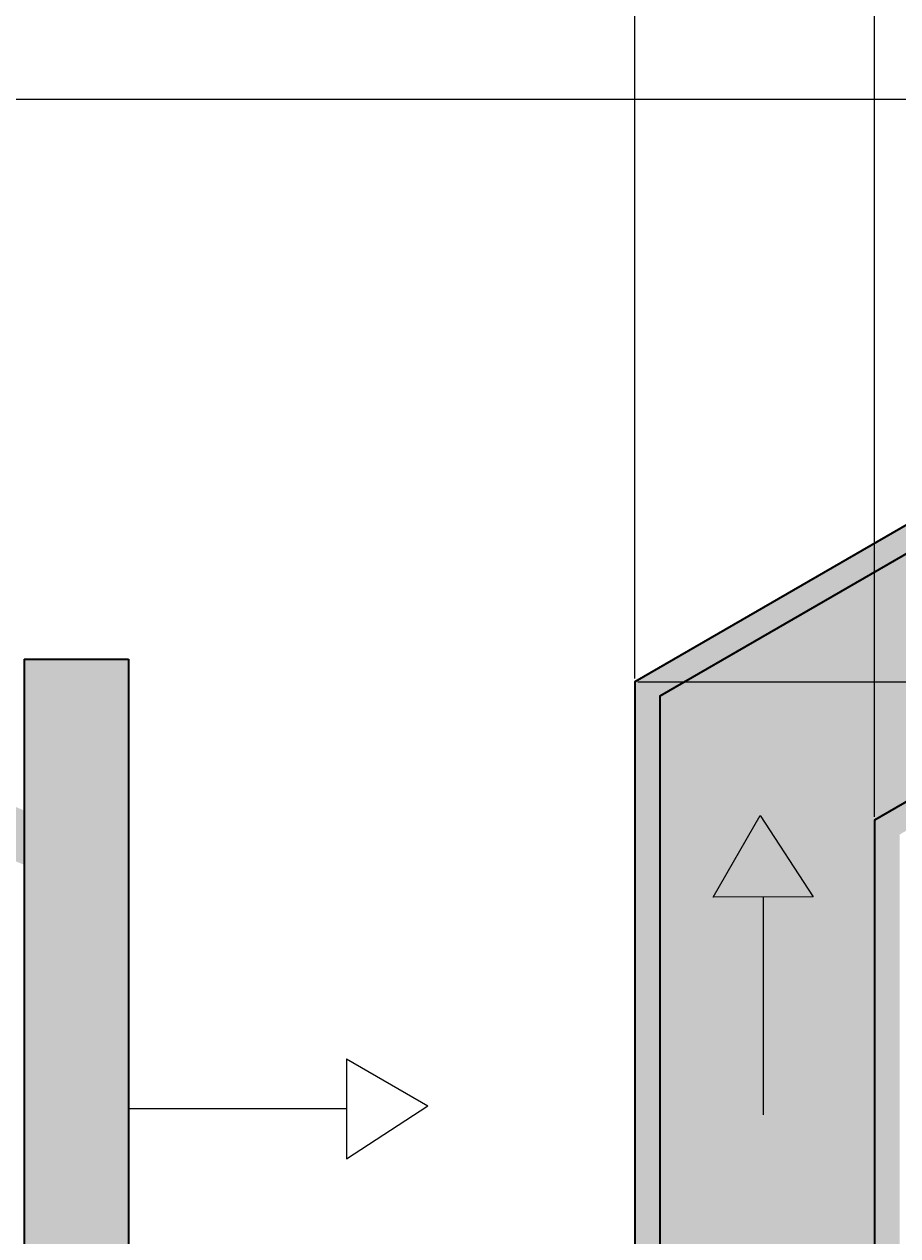
# Model space of a CAD drawing. Units: inches. Extents: x -1 to 292, y -3 to 199.
# Tile 41 of 52: x 203.03 to 220.5, y 77.05 to 101.27. Entities that reach past the tile are written whole.
import ezdxf

# ---------------------------------------------------------------- set-up
doc = ezdxf.new("R2010")
doc.units = ezdxf.units.IN
doc.header["$MEASUREMENT"] = 0
for name, color, linetype, lineweight in [('M-ANNO-SYMB', 1, 'Continuous', 18), ('M-DIMS', 2, 'Continuous', 18), ('M-EQPM', 7, 'Continuous', 35), ('M-PATT', 8, 'Continuous', 13)]:
    doc.layers.add(name, color=color, linetype=linetype, lineweight=lineweight)
doc.styles.get("Standard").update_dxf_attribs({"font": 'arial.ttf'})
doc.dimstyles.get("Standard").update_dxf_attribs({"dimtxt": 0.18, "dimasz": 0.18, "dimexe": 0.18, "dimexo": 0.0625, "dimgap": 0.09, "dimtad": 0, "dimtih": 1, "dimtoh": 1, "dimdec": 4, "dimzin": 0, "dimdsep": 46, "dimtxsty": 'Standard', "dimcen": 0.09, "dimadec": 0, "dimazin": 0, "dimtfac": 1, "dimtdec": 4, "dimtofl": 0, "dimtmove": 0, "dimatfit": 3, "dimfxl": 1, "dimtolj": 1, "dimtzin": 0, "dimarcsym": 0})

# ---------------------------------------------------------------- blocks, each defined once
blk = doc.blocks.new('FLOW-ARROW-GAS')
for p, q in [((201.507, 38.14), (201.507, 36.14)), ((201.507, 38.14), (203.137, 37.199)), ((201.507, 37.14), (197.151, 37.14)), ((201.507, 36.14), (203.137, 37.199))]:
    blk.add_line(p, q)
blk = doc.blocks.new('FLOW-ARROW-WATER')
blk.add_line((223.29, 53.741), (227.063, 51.564))
blk.add_lwpolyline([(222.79, 52.875), (221.849, 54.506), (223.79, 54.608)], close=True)
blk = doc.blocks.new('DUCT-FLANGE')
for p, q in [((0, 34), (0, 0)), ((0, 34), (2.089, 34)), ((2.089, 34), (2.089, 0))]:
    blk.add_line(p, q)
blk = doc.blocks.new('*D10')
at = {"layer": 'Defpoints', "color": 0, "transparency": 16777216}
for p in [(169.176, 99.774), (169.176, 43.391), (292.04, 43.391)]:
    blk.add_point(p, dxfattribs=at)
at = {"layer": 'M-DIMS', "color": 0, "lineweight": -2, "transparency": 16777216}
for p, q in [((169.239, 99.774), (292.22, 99.774)), ((292.04, 99.594), (292.04, 71.764)), ((292.04, 43.571), (292.04, 71.4)), ((169.239, 43.391), (292.22, 43.391))]:
    blk.add_line(p, q, dxfattribs=at)
at = {"layer": 'M-DIMS', "color": 0, "transparency": 16777216}
for points in [[(292.01, 99.594), (292.07, 99.594), (292.04, 99.774)], [(292.01, 43.571), (292.07, 43.571), (292.04, 43.391)]]:
    blk.add_solid(points, dxfattribs=at)
at = {"layer": 'M-DIMS', "color": 0, "transparency": 16777216, "insert": (292.04, 71.582), "char_height": 0.18, "attachment_point": 5}
blk.add_mtext('\\A1;56.38', dxfattribs=at)
blk = doc.blocks.new('*D25')
at = {"layer": 'Defpoints', "color": 0, "transparency": 16777216}
for p in [(273.066, 88.419), (215.241, 88.13), (273.066, -2.71)]:
    blk.add_point(p, dxfattribs=at)
at = {"layer": 'M-DIMS', "color": 0, "lineweight": -2, "transparency": 16777216}
for p, q in [((273.066, 88.357), (273.066, -2.89)), ((215.241, 88.068), (215.241, -2.89)), ((215.421, -2.71), (243.76, -2.71)), ((272.886, -2.71), (244.547, -2.71))]:
    blk.add_line(p, q, dxfattribs=at)
at = {"layer": 'M-DIMS', "color": 0, "transparency": 16777216}
for points in [[(215.421, -2.68), (215.421, -2.74), (215.241, -2.71)], [(272.886, -2.68), (272.886, -2.74), (273.066, -2.71)]]:
    blk.add_solid(points, dxfattribs=at)
at = {"layer": 'M-DIMS', "color": 0, "transparency": 16777216, "insert": (244.153, -2.71), "char_height": 0.18, "attachment_point": 5}
blk.add_mtext('\\A1;57.83', dxfattribs=at)
blk = doc.blocks.new('*D26')
at = {"layer": 'Defpoints', "color": 0, "transparency": 16777216}
for p in [(215.241, 88.13), (215.241, 55.034), (229.841, 55.034)]:
    blk.add_point(p, dxfattribs=at)
at = {"layer": 'M-DIMS', "color": 0, "lineweight": -2, "transparency": 16777216}
for p, q in [((215.303, 88.13), (230.021, 88.13)), ((229.841, 87.95), (229.841, 71.764)), ((229.841, 55.214), (229.841, 71.4)), ((215.303, 55.034), (230.021, 55.034))]:
    blk.add_line(p, q, dxfattribs=at)
at = {"layer": 'M-DIMS', "color": 0, "transparency": 16777216}
for points in [[(229.811, 87.95), (229.871, 87.95), (229.841, 88.13)], [(229.811, 55.214), (229.871, 55.214), (229.841, 55.034)]]:
    blk.add_solid(points, dxfattribs=at)
at = {"layer": 'M-DIMS', "color": 0, "transparency": 16777216, "insert": (229.841, 71.582), "char_height": 0.18, "attachment_point": 5}
blk.add_mtext('\\A1;33.1', dxfattribs=at)
blk = doc.blocks.new('*D27')
at = {"layer": 'Defpoints', "color": 0, "transparency": 16777216}
for p in [(220.034, 174.363), (215.241, 88.13), (220.034, 85.363)]:
    blk.add_point(p, dxfattribs=at)
at = {"layer": 'M-DIMS', "color": 0, "lineweight": -2, "transparency": 16777216}
for p, q in [((215.241, 88.193), (215.241, 174.543)), ((220.034, 85.426), (220.034, 174.543)), ((215.421, 174.363), (217.24, 174.363)), ((219.854, 174.363), (218.035, 174.363))]:
    blk.add_line(p, q, dxfattribs=at)
at = {"layer": 'M-DIMS', "color": 0, "transparency": 16777216}
for points in [[(215.421, 174.393), (215.421, 174.333), (215.241, 174.363)], [(219.854, 174.393), (219.854, 174.333), (220.034, 174.363)]]:
    blk.add_solid(points, dxfattribs=at)
at = {"layer": 'M-DIMS', "color": 0, "transparency": 16777216, "insert": (217.637, 174.363), "char_height": 0.18, "attachment_point": 5}
blk.add_mtext('\\A1;4.793', dxfattribs=at)

msp = doc.modelspace()

# ---------------------------------------------------------------- hatches: boundary and pattern name
at = {"layer": 'M-PATT'}
h = msp.add_hatch(color=256, dxfattribs=at)
h.set_gradient(color1=(0, 255, 255), color2=(0, 255, 255), tint=1, name='CYLINDER')
h.paths.add_polyline_path([(256.8092, 99.5764), (256.4077, 99.3157), (253.7155, 100.87), (251.3221, 99.3157), (248.6299, 100.87), (246.2365, 99.3157), (243.5443, 100.87), (241.1509, 99.3157), (238.4587, 100.87), (236.4209, 99.5466), (236.4209, 97.1861), (234.9209, 97.1861), (234.9209, 99.9764), (233.3731, 100.87), (230.9797, 99.3157, 1.0704128)])
h.paths.add_polyline_path([(234.4549, 44.5975, 1), (253.3518, 44.5975, 1)])
h.paths.add_polyline_path([(235.4822, 48.8821), (220.034, 57.8011), (220.034, 85.363), (232.4507, 92.5318, -0.0853739), (231.0925, 96.7051), (215.7407, 87.8418), (215.7407, 55.3224), (234.4552, 44.5176, -0.0021162), (234.4549, 44.5975, -0.1182098)])
h.paths.add_polyline_path([(222.7904, 52.8755), (221.8492, 54.5058), (223.7904, 54.6075)], flags=16)
h.paths.add_polyline_path([(216.828, 66.8912), (217.7692, 68.5216), (218.828, 66.8912)], flags=16)
h.paths.add_polyline_path([(216.8084, 83.826), (217.7497, 85.4564), (218.8084, 83.826)], flags=16)
h.paths.add_polyline_path([(226.468, 92.8803), (228.3442, 93.0348), (227.6068, 91.2362)], flags=16)
h.paths.add_polyline_path([(272.5659, 88.1304), (260.2765, 95.2257), (259.0113, 93.0196), (263.0639, 91.1046), (263.4912, 92.0087), (264.5631, 90.4612), (262.6367, 90.2004), (263.0639, 91.1046), (259.0113, 93.0196), (257.8918, 91.0677), (267.7726, 85.363), (267.7726, 57.8011), (255.5043, 50.718), (257.0663, 46.085), (272.5659, 55.0337)])
h.paths.add_polyline_path([(263.6286, 51.5636), (261.7461, 51.5636), (262.6286, 53.2956)], flags=16)
h.paths.add_polyline_path([(269.8773, 65.3608), (268.8186, 66.9911), (270.8186, 66.9911)], flags=16)
h.paths.add_polyline_path([(269.8773, 80.8843), (268.8186, 82.5146), (270.8186, 82.5146)], flags=16)
h.paths.add_polyline_path([(255.5043, 50.718), (252.3244, 48.8821, -0.1182098), (253.3518, 44.5975, -0.0177685), (253.3279, 43.9266), (257.0663, 46.085)])
h.paths.add_polyline_path([(260.2765, 95.2257), (256.7809, 97.2439, -0.0959457), (255.356, 92.5318), (257.8918, 91.0677)])
h = msp.add_hatch(color=256, dxfattribs=at)
h.set_gradient(color1=(76, 38, 47), color2=(76, 38, 47), tint=1, name='CYLINDER')
h.paths.add_polyline_path([(267.2726, 58.0898), (255.3414, 51.2013), (255.5043, 50.718), (267.7726, 57.8011), (267.7726, 85.363), (257.8918, 91.0677), (257.643, 90.634), (267.2726, 85.0743)])
h.paths.add_polyline_path([(272.5659, 55.0337), (257.0663, 46.085), (257.2293, 45.6017), (273.0659, 54.745), (273.0659, 88.4191), (260.5253, 95.6595), (260.2765, 95.2257), (272.5659, 88.1304)])
h.paths.add_polyline_path([(215.2407, 55.0337), (234.4787, 43.9266, -0.0156517), (234.4552, 44.5176), (215.7407, 55.3224), (215.7407, 87.8418), (231.0925, 96.7051, -0.0104859), (231.0257, 97.2439), (215.2407, 88.1304)])
h.paths.add_polyline_path([(220.034, 57.8011), (235.4822, 48.8821, -0.0132367), (235.7207, 49.3218), (220.534, 58.0898), (220.534, 85.0743), (232.6923, 92.0939, -0.0096587), (232.4507, 92.5318), (220.034, 85.363)])
h = msp.add_hatch(color=256, dxfattribs=at)
h.set_gradient(color1=(76, 38, 47), color2=(76, 38, 47), tint=1, name='CYLINDER')
h.paths.add_polyline_path([(40.8628, 91.6478), (40.3591, 92.5203), (23.9502, 85.5552), (23.9502, 84.4688)])
h.paths.add_polyline_path([(52.8586, 93.6403), (42.9977, 93.6403), (40.3591, 92.5203), (40.8628, 91.6478), (43.2011, 92.6403), (54.4604, 92.6403, -0.0601508)])
h.paths.add_polyline_path([(23.9502, 88.5821), (21.8612, 88.5821), (21.8612, 54.5821), (23.9502, 54.5821)])
h.paths.add_polyline_path([(23.9502, 58.376), (23.9502, 57.2213), (42.9332, 46.2615), (50.4659, 46.2615, -0.0351813), (50.9409, 47.2615), (43.2011, 47.2615)])
h.paths.add_polyline_path([(179.5897, 93.6403), (174.1181, 93.6403, -0.0601508), (172.5163, 92.6403), (179.5897, 92.6403)])
h.paths.add_polyline_path([(183.979, 93.6403), (181.5897, 93.6403), (181.5897, 92.6403), (183.7755, 92.6403), (203.0265, 84.4688), (203.0265, 85.5552)])
h.paths.add_polyline_path([(205.1155, 88.5821), (203.0265, 88.5821), (203.0265, 54.5821), (205.1155, 54.5821)])
h.paths.add_polyline_path([(203.0265, 57.2213), (203.0265, 58.376), (183.7755, 47.2615), (181.5897, 47.2615), (181.5897, 46.2615), (184.0435, 46.2615)])
h.paths.add_polyline_path([(179.5897, 47.2615), (176.0358, 47.2615, -0.0351813), (176.5107, 46.2615), (179.5897, 46.2615)])
h = msp.add_hatch(color=256, dxfattribs=at)
h.set_gradient(color1=(0, 0, 255), color2=(0, 0, 255), tint=1, name='CYLINDER')
h.paths.add_polyline_path([(227.6068, 91.2362), (228.3442, 93.0348), (226.468, 92.8803)])
h.paths.add_polyline_path([(218.8084, 83.826), (217.7497, 85.4564), (216.8084, 83.826)])
h.paths.add_polyline_path([(262.6367, 90.2004), (264.5631, 90.4612), (263.4912, 92.0087)])
h.paths.add_polyline_path([(217.7692, 68.5216), (216.828, 66.8912), (218.828, 66.8912)])
h.paths.add_polyline_path([(223.7904, 54.6075), (221.8492, 54.5058), (222.7904, 52.8755)])
h.paths.add_polyline_path([(262.6286, 53.2956), (261.7461, 51.5636), (263.6286, 51.5636)])
h.paths.add_polyline_path([(268.8186, 82.5146), (269.8773, 80.8843), (270.8186, 82.5146)])
h.paths.add_polyline_path([(268.8186, 66.9911), (269.8773, 65.3608), (270.8186, 66.9911)])

# ---------------------------------------------------------------- linework, layer by layer
at = {"layer": 'M-EQPM'}
for points in [[(231.0257, 97.2439), (215.2407, 88.1304), (215.2407, 55.0337), (234.4787, 43.9266)], [(231.0925, 96.7051), (215.7407, 87.8418), (215.7407, 55.3224), (234.4552, 44.5176)], [(232.4507, 92.5318), (220.034, 85.363), (220.034, 57.8011), (235.4822, 48.8821)]]:
    msp.add_lwpolyline(points, dxfattribs=at)

# ---------------------------------------------------------------- block references
at = {"layer": 'M-ANNO-SYMB', "rotation": 300.0000000000007}
msp.add_blockref('FLOW-ARROW-WATER', (59.6217, 250.3305), dxfattribs=at)
at = {"layer": 'M-ANNO-SYMB'}
msp.add_blockref('FLOW-ARROW-GAS', (7.9644, 42.4546), dxfattribs=at)
at = {"layer": 'M-EQPM'}
msp.add_blockref('DUCT-FLANGE', (203.0263, 54.582), dxfattribs=at)

# ---------------------------------------------------------------- dimensions: what is measured, and where the dimension line sits
at = {"layer": 'M-DIMS'}
for base, p2, override, picture, middle in [((220.034, 174.3627), (220.034, 85.363), {"dimdec": 3, "dimlfac": 1, "dimrnd": 0, "dimzin": 0, "dimdsep": 46, "dimlunit": 2}, '*D27', (217.6374, 174.3627)), ((273.0659, -2.7104), (273.0659, 88.4191), {"dimdec": 2, "dimlfac": 1, "dimrnd": 0, "dimzin": 0, "dimdsep": 46, "dimlunit": 2}, '*D25', (244.1533, -2.7104))]:
    dim = msp.add_linear_dim(base=base, p1=(215.2407, 88.1304), p2=p2, dimstyle='Standard', override=override, dxfattribs=at)
    dim.commit()
    dim.dimension.update_dxf_attribs({"geometry": picture, "text_midpoint": middle})
for base, p1, p2, angle, override, picture, middle in [((292.0399, 43.3906), (169.176, 99.7735), (169.176, 43.3906), 90, {"dimdec": 2, "dimlfac": 1, "dimrnd": 0, "dimzin": 0, "dimdsep": 46, "dimlunit": 2}, '*D10', (292.0399, 71.5821)), ((229.8407, 55.0337), (215.2407, 88.1304), (215.2407, 55.0337), 270, {"dimdec": 1, "dimlfac": 1, "dimrnd": 0, "dimzin": 0, "dimdsep": 46, "dimlunit": 2}, '*D26', (229.8407, 71.5821))]:
    dim = msp.add_linear_dim(base=base, p1=p1, p2=p2, angle=angle, dimstyle='Standard', override=override, dxfattribs=at)
    dim.commit()
    dim.dimension.update_dxf_attribs({"geometry": picture, "text_midpoint": middle})

doc.saveas('drawing.dxf')
